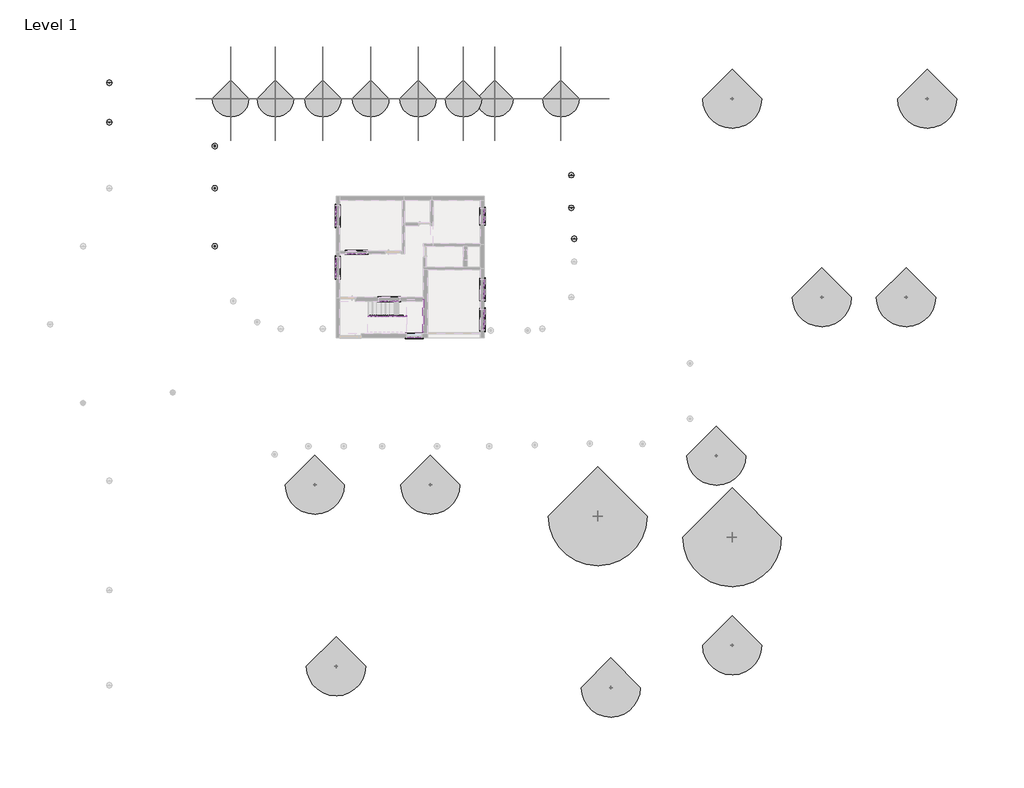
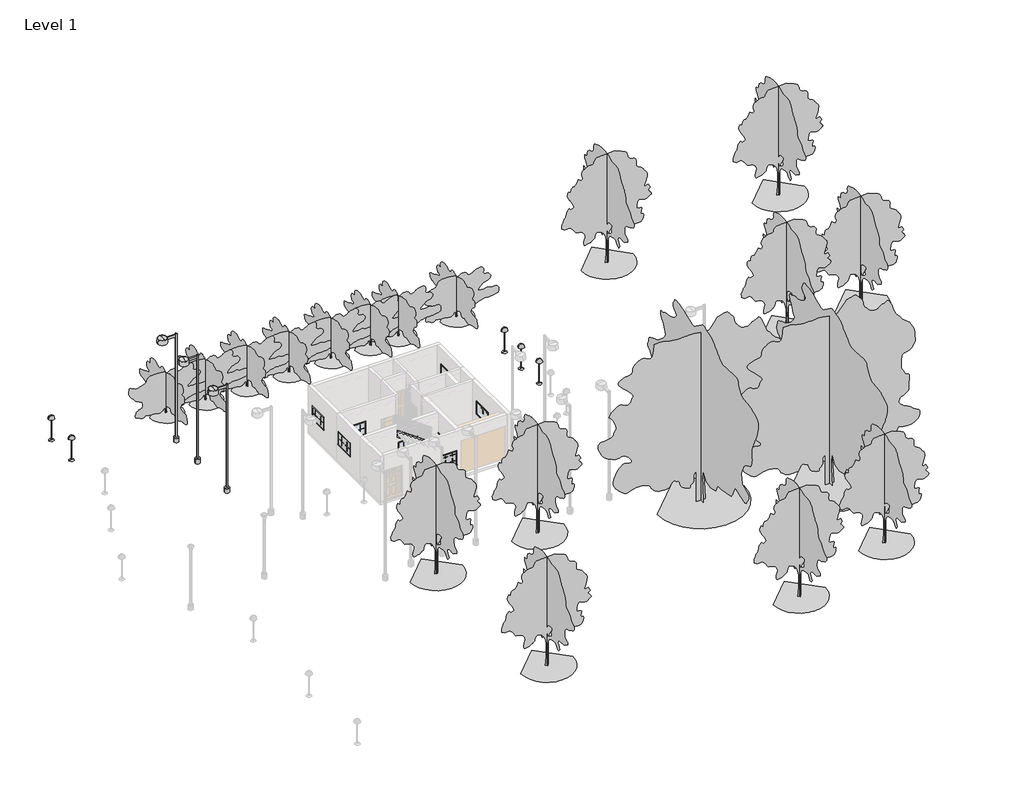
# One storey, part 3 of 3: 36 proxies, 20 geographic elements, 8 light fixtures, 4 members.
"""IFC4 building model written with IfcOpenShell, lengths in millimetres."""

from ifc_helpers import new_model, si_unit, frame, origin, place, context, project, spatial, polyline, outline, extrude, transform, mapped, element, save
from components import m_muntin_pattern_2x2_m_muntin_pattern_2x2_8d9e5da3, m_muntin_pattern_2x2_m_muntin_pattern_2x2_32a0f80e, m_muntin_pattern_2x2_m_muntin_pattern_2x2_5c9fa27a, m_muntin_pattern_2x2_m_muntin_pattern_2x2_8c7fd3cb, m_muntin_pattern_2x2_m_muntin_pattern_2x2_332c70e0, m_trim_window_exterior_flat_with_sill_3a557199, m_trim_window_exterior_flat_with_sill_8fa486dc, m_trim_window_interior_flat_picture_frame_580345df, m_trim_window_interior_flat_picture_frame_b6dd03a6, m_rpc_tree_deciduous_kousa_dogwood_3_0_meters_e0625334, m_rpc_tree_deciduous_largetooth_aspen_7_6_meters_a2efc43f, m_rpc_tree_deciduous_scarlet_oak_12_5_meters_78a4568a, m_floor_lamp_hemispheric_60w_120v_4a08ccbb, m_street_light_standard_250w_halogen_480v_204dbcbb

model = new_model("IFC4")

# Units and contexts
model_context = context("Model", 3, world=origin())
ifc_project = project(units=[si_unit("LENGTHUNIT", "METRE", prefix="MILLI")], contexts=[model_context])

# Site, building, storey
site = spatial("IfcSite", under=ifc_project)
building = spatial("IfcBuilding", under=site)
storey = spatial("IfcBuildingStorey", under=building, Name="Level 1", Elevation=0.0)

# Proxies
placement = place(None, origin())
m_muntin_pattern_2x2_m_muntin_pattern_2x2_shape = m_muntin_pattern_2x2_m_muntin_pattern_2x2_8d9e5da3(model_context)
element("IfcBuildingElementProxy", 1, Name="M_Muntin Pattern_2x2 : M_Muntin Pattern_2x2", ObjectType="M_Muntin Pattern_2x2 : M_Muntin Pattern_2x2", at=placement, inside=storey, context=model_context, shape_type="MappedRepresentation", body=[
    mapped(m_muntin_pattern_2x2_m_muntin_pattern_2x2_shape, transform((-8281.8157945, -2418.5171603, 1289.05), x_axis=(-1.0, 0.0, 0.0), y_axis=(0.0, -1.0, 0.0), z_axis=(0.0, 0.0, 1.0))),
])
element("IfcBuildingElementProxy", 2, Name="M_Muntin Pattern_2x2 : M_Muntin Pattern_2x2", ObjectType="M_Muntin Pattern_2x2 : M_Muntin Pattern_2x2", at=placement, inside=storey, context=model_context, shape_type="MappedRepresentation", body=[
    mapped(m_muntin_pattern_2x2_m_muntin_pattern_2x2_shape, transform((-3082.7532945, -3204.3296603, 1289.05), x_axis=(0.0, -1.0, 0.0), y_axis=(1.0, 0.0, 0.0), z_axis=(0.0, 0.0, 1.0))),
])
element("IfcBuildingElementProxy", 3, Name="M_Muntin Pattern_2x2 : M_Muntin Pattern_2x2", ObjectType="M_Muntin Pattern_2x2 : M_Muntin Pattern_2x2", at=placement, inside=storey, context=model_context, shape_type="MappedRepresentation", body=[
    mapped(m_muntin_pattern_2x2_m_muntin_pattern_2x2_shape, transform((-3082.7532945, -1461.6515353, 1289.05), x_axis=(0.0, -1.0, 0.0), y_axis=(1.0, 0.0, 0.0), z_axis=(0.0, 0.0, 1.0))),
])
element("IfcBuildingElementProxy", 4, Name="M_Muntin Pattern_2x2 : M_Muntin Pattern_2x2", ObjectType="M_Muntin Pattern_2x2 : M_Muntin Pattern_2x2", at=placement, inside=storey, context=model_context, shape_type="MappedRepresentation", body=[
    mapped(m_muntin_pattern_2x2_m_muntin_pattern_2x2_shape, transform((-11648.9032945, 2196.3453397, 1289.05), x_axis=(0.0, 1.0, 0.0), y_axis=(-1.0, 0.0, 0.0), z_axis=(0.0, 0.0, 1.0))),
])
element("IfcBuildingElementProxy", 5, Name="M_Muntin Pattern_2x2 : M_Muntin Pattern_2x2", ObjectType="M_Muntin Pattern_2x2 : M_Muntin Pattern_2x2", at=placement, inside=storey, context=model_context, shape_type="MappedRepresentation", body=[
    mapped(m_muntin_pattern_2x2_m_muntin_pattern_2x2_shape, transform((-11648.9032945, -800.8546603, 1289.05), x_axis=(0.0, 1.0, 0.0), y_axis=(-1.0, 0.0, 0.0), z_axis=(0.0, 0.0, 1.0))),
])
element("IfcBuildingElementProxy", 6, Name="M_Muntin Pattern_2x2 : M_Muntin Pattern_2x2", ObjectType="M_Muntin Pattern_2x2 : M_Muntin Pattern_2x2", at=placement, inside=storey, context=model_context, shape_type="MappedRepresentation", body=[
    mapped(m_muntin_pattern_2x2_m_muntin_pattern_2x2_shape, transform((-10165.3845445, 324.6828397, 1289.05), x_axis=(-1.0, 0.0, 0.0), y_axis=(0.0, -1.0, 0.0), z_axis=(0.0, 0.0, 1.0))),
])
m_muntin_pattern_2x2_m_muntin_pattern_2x2_2_shape = m_muntin_pattern_2x2_m_muntin_pattern_2x2_32a0f80e(model_context)
element("IfcBuildingElementProxy", 7, Name="M_Muntin Pattern_2x2 : M_Muntin Pattern_2x2", ObjectType="M_Muntin Pattern_2x2 : M_Muntin Pattern_2x2", at=placement, inside=storey, context=model_context, shape_type="MappedRepresentation", body=[
    mapped(m_muntin_pattern_2x2_m_muntin_pattern_2x2_2_shape, transform((-8888.2407945, -2418.5171603, 1289.05), x_axis=(1.0, 0.0, 0.0), y_axis=(0.0, 1.0, 0.0), z_axis=(0.0, 0.0, 1.0))),
])
element("IfcBuildingElementProxy", 8, Name="M_Muntin Pattern_2x2 : M_Muntin Pattern_2x2", ObjectType="M_Muntin Pattern_2x2 : M_Muntin Pattern_2x2", at=placement, inside=storey, context=model_context, shape_type="MappedRepresentation", body=[
    mapped(m_muntin_pattern_2x2_m_muntin_pattern_2x2_2_shape, transform((-3082.7532945, -3810.7546603, 1289.05), x_axis=(0.0, 1.0, 0.0), y_axis=(-1.0, 0.0, 0.0), z_axis=(0.0, 0.0, 1.0))),
])
element("IfcBuildingElementProxy", 9, Name="M_Muntin Pattern_2x2 : M_Muntin Pattern_2x2", ObjectType="M_Muntin Pattern_2x2 : M_Muntin Pattern_2x2", at=placement, inside=storey, context=model_context, shape_type="MappedRepresentation", body=[
    mapped(m_muntin_pattern_2x2_m_muntin_pattern_2x2_2_shape, transform((-3082.7532945, -2068.0765353, 1289.05), x_axis=(0.0, 1.0, 0.0), y_axis=(-1.0, 0.0, 0.0), z_axis=(0.0, 0.0, 1.0))),
])
element("IfcBuildingElementProxy", 10, Name="M_Muntin Pattern_2x2 : M_Muntin Pattern_2x2", ObjectType="M_Muntin Pattern_2x2 : M_Muntin Pattern_2x2", at=placement, inside=storey, context=model_context, shape_type="MappedRepresentation", body=[
    mapped(m_muntin_pattern_2x2_m_muntin_pattern_2x2_2_shape, transform((-11648.9032945, 2802.7703397, 1289.05), x_axis=(0.0, -1.0, 0.0), y_axis=(1.0, 0.0, 0.0), z_axis=(0.0, 0.0, 1.0))),
])
element("IfcBuildingElementProxy", 11, Name="M_Muntin Pattern_2x2 : M_Muntin Pattern_2x2", ObjectType="M_Muntin Pattern_2x2 : M_Muntin Pattern_2x2", at=placement, inside=storey, context=model_context, shape_type="MappedRepresentation", body=[
    mapped(m_muntin_pattern_2x2_m_muntin_pattern_2x2_2_shape, transform((-11648.9032945, -194.4296603, 1289.05), x_axis=(0.0, -1.0, 0.0), y_axis=(1.0, 0.0, 0.0), z_axis=(0.0, 0.0, 1.0))),
])
element("IfcBuildingElementProxy", 12, Name="M_Muntin Pattern_2x2 : M_Muntin Pattern_2x2", ObjectType="M_Muntin Pattern_2x2 : M_Muntin Pattern_2x2", at=placement, inside=storey, context=model_context, shape_type="MappedRepresentation", body=[
    mapped(m_muntin_pattern_2x2_m_muntin_pattern_2x2_2_shape, transform((-10771.8095445, 324.6828397, 1289.05), x_axis=(1.0, 0.0, 0.0), y_axis=(0.0, 1.0, 0.0), z_axis=(0.0, 0.0, 1.0))),
])
m_muntin_pattern_2x2_m_muntin_pattern_2x2_3_shape = m_muntin_pattern_2x2_m_muntin_pattern_2x2_5c9fa27a(model_context)
element("IfcBuildingElementProxy", 13, Name="M_Muntin Pattern_2x2 : M_Muntin Pattern_2x2", ObjectType="M_Muntin Pattern_2x2 : M_Muntin Pattern_2x2", at=placement, inside=storey, context=model_context, shape_type="MappedRepresentation", body=[
    mapped(m_muntin_pattern_2x2_m_muntin_pattern_2x2_3_shape, transform((-6910.2157945, -4552.1171603, 984.25), x_axis=(-1.0, 0.0, 0.0), y_axis=(0.0, -1.0, 0.0), z_axis=(0.0, 0.0, 1.0))),
])
element("IfcBuildingElementProxy", 14, Name="M_Muntin Pattern_2x2 : M_Muntin Pattern_2x2", ObjectType="M_Muntin Pattern_2x2 : M_Muntin Pattern_2x2", at=placement, inside=storey, context=model_context, shape_type="MappedRepresentation", body=[
    mapped(m_muntin_pattern_2x2_m_muntin_pattern_2x2_3_shape, transform((-3082.7532945, 2701.1703397, 1289.05), x_axis=(0.0, -1.0, 0.0), y_axis=(1.0, 0.0, 0.0), z_axis=(0.0, 0.0, 1.0))),
])
m_muntin_pattern_2x2_m_muntin_pattern_2x2_4_shape = m_muntin_pattern_2x2_m_muntin_pattern_2x2_8c7fd3cb(model_context)
element("IfcBuildingElementProxy", 15, Name="M_Muntin Pattern_2x2 : M_Muntin Pattern_2x2", ObjectType="M_Muntin Pattern_2x2 : M_Muntin Pattern_2x2", at=placement, inside=storey, context=model_context, shape_type="MappedRepresentation", body=[
    mapped(m_muntin_pattern_2x2_m_muntin_pattern_2x2_4_shape, transform((-7364.2407945, -4552.1171603, 984.25), x_axis=(1.0, 0.0, 0.0), y_axis=(0.0, 1.0, 0.0), z_axis=(0.0, 0.0, 1.0))),
])
element("IfcBuildingElementProxy", 16, Name="M_Muntin Pattern_2x2 : M_Muntin Pattern_2x2", ObjectType="M_Muntin Pattern_2x2 : M_Muntin Pattern_2x2", at=placement, inside=storey, context=model_context, shape_type="MappedRepresentation", body=[
    mapped(m_muntin_pattern_2x2_m_muntin_pattern_2x2_4_shape, transform((-3082.7532945, 2247.1453397, 1289.05), x_axis=(0.0, 1.0, 0.0), y_axis=(-1.0, 0.0, 0.0), z_axis=(0.0, 0.0, 1.0))),
])
m_muntin_pattern_2x2_m_muntin_pattern_2x2_5_shape = m_muntin_pattern_2x2_m_muntin_pattern_2x2_332c70e0(model_context)
element("IfcBuildingElementProxy", 17, Name="M_Muntin Pattern_2x2 : M_Muntin Pattern_2x2", ObjectType="M_Muntin Pattern_2x2 : M_Muntin Pattern_2x2", at=placement, inside=storey, context=model_context, shape_type="MappedRepresentation", body=[
    mapped(m_muntin_pattern_2x2_m_muntin_pattern_2x2_5_shape, transform((-7364.2407945, -4552.1171603, 1584.25), x_axis=(1.0, 0.0, 0.0), y_axis=(0.0, 1.0, 0.0), z_axis=(0.0, 0.0, 1.0))),
])
element("IfcBuildingElementProxy", 18, Name="M_Muntin Pattern_2x2 : M_Muntin Pattern_2x2", ObjectType="M_Muntin Pattern_2x2 : M_Muntin Pattern_2x2", at=placement, inside=storey, context=model_context, shape_type="MappedRepresentation", body=[
    mapped(m_muntin_pattern_2x2_m_muntin_pattern_2x2_5_shape, transform((-6910.2157945, -4552.1171603, 1584.25), x_axis=(1.0, 0.0, 0.0), y_axis=(0.0, 1.0, 0.0), z_axis=(0.0, 0.0, 1.0))),
])
element("IfcBuildingElementProxy", 19, Name="M_Muntin Pattern_2x2 : M_Muntin Pattern_2x2", ObjectType="M_Muntin Pattern_2x2 : M_Muntin Pattern_2x2", at=placement, inside=storey, context=model_context, shape_type="MappedRepresentation", body=[
    mapped(m_muntin_pattern_2x2_m_muntin_pattern_2x2_5_shape, transform((-3082.7532945, 2247.1453397, 1889.05), x_axis=(0.0, 1.0, 0.0), y_axis=(-1.0, 0.0, 0.0), z_axis=(0.0, 0.0, 1.0))),
])
element("IfcBuildingElementProxy", 20, Name="M_Muntin Pattern_2x2 : M_Muntin Pattern_2x2", ObjectType="M_Muntin Pattern_2x2 : M_Muntin Pattern_2x2", at=placement, inside=storey, context=model_context, shape_type="MappedRepresentation", body=[
    mapped(m_muntin_pattern_2x2_m_muntin_pattern_2x2_5_shape, transform((-3082.7532945, 2701.1703397, 1889.05), x_axis=(0.0, 1.0, 0.0), y_axis=(-1.0, 0.0, 0.0), z_axis=(0.0, 0.0, 1.0))),
])
m_trim_window_exterior_flat_with_sill_shape = m_trim_window_exterior_flat_with_sill_3a557199(model_context)
element("IfcBuildingElementProxy", 21, Name="M_Trim-Window-Exterior-Flat : with Sill", ObjectType="M_Trim-Window-Exterior-Flat : with Sill", at=placement, inside=storey, context=model_context, shape_type="MappedRepresentation", body=[
    mapped(m_trim_window_exterior_flat_with_sill_shape, transform((-8585.0282945, -2428.0421603, 2019.2), x_axis=(1.0, 0.0, 0.0), y_axis=(0.0, 0.0, 1.0), z_axis=(0.0, -1.0, 0.0))),
])
element("IfcBuildingElementProxy", 22, Name="M_Trim-Window-Exterior-Flat : with Sill", ObjectType="M_Trim-Window-Exterior-Flat : with Sill", at=placement, inside=storey, context=model_context, shape_type="MappedRepresentation", body=[
    mapped(m_trim_window_exterior_flat_with_sill_shape, transform((-3073.2282945, -3507.5421603, 2019.2), x_axis=(0.0, 1.0, 0.0), y_axis=(0.0, 0.0, 1.0), z_axis=(1.0, 0.0, 0.0))),
])
element("IfcBuildingElementProxy", 23, Name="M_Trim-Window-Exterior-Flat : with Sill", ObjectType="M_Trim-Window-Exterior-Flat : with Sill", at=placement, inside=storey, context=model_context, shape_type="MappedRepresentation", body=[
    mapped(m_trim_window_exterior_flat_with_sill_shape, transform((-3073.2282945, -1764.8640353, 2019.2), x_axis=(0.0, 1.0, 0.0), y_axis=(0.0, 0.0, 1.0), z_axis=(1.0, 0.0, 0.0))),
])
element("IfcBuildingElementProxy", 24, Name="M_Trim-Window-Exterior-Flat : with Sill", ObjectType="M_Trim-Window-Exterior-Flat : with Sill", at=placement, inside=storey, context=model_context, shape_type="MappedRepresentation", body=[
    mapped(m_trim_window_exterior_flat_with_sill_shape, transform((-11658.4282945, 2499.5578397, 2019.2), x_axis=(0.0, -1.0, 0.0), y_axis=(0.0, 0.0, 1.0), z_axis=(-1.0, 0.0, 0.0))),
])
element("IfcBuildingElementProxy", 25, Name="M_Trim-Window-Exterior-Flat : with Sill", ObjectType="M_Trim-Window-Exterior-Flat : with Sill", at=placement, inside=storey, context=model_context, shape_type="MappedRepresentation", body=[
    mapped(m_trim_window_exterior_flat_with_sill_shape, transform((-11658.4282945, -497.6421603, 2019.2), x_axis=(0.0, -1.0, 0.0), y_axis=(0.0, 0.0, 1.0), z_axis=(-1.0, 0.0, 0.0))),
])
element("IfcBuildingElementProxy", 26, Name="M_Trim-Window-Exterior-Flat : with Sill", ObjectType="M_Trim-Window-Exterior-Flat : with Sill", at=placement, inside=storey, context=model_context, shape_type="MappedRepresentation", body=[
    mapped(m_trim_window_exterior_flat_with_sill_shape, transform((-10468.5970445, 315.1578397, 2019.2), x_axis=(1.0, 0.0, 0.0), y_axis=(0.0, 0.0, 1.0), z_axis=(0.0, -1.0, 0.0))),
])
m_trim_window_exterior_flat_with_sill_2_shape = m_trim_window_exterior_flat_with_sill_8fa486dc(model_context)
element("IfcBuildingElementProxy", 27, Name="M_Trim-Window-Exterior-Flat : with Sill", ObjectType="M_Trim-Window-Exterior-Flat : with Sill", at=placement, inside=storey, context=model_context, shape_type="MappedRepresentation", body=[
    mapped(m_trim_window_exterior_flat_with_sill_2_shape, transform((-7137.2282945, -4561.6421603, 1814.4), x_axis=(1.0, 0.0, 0.0), y_axis=(0.0, 0.0, 1.0), z_axis=(0.0, -1.0, 0.0))),
])
element("IfcBuildingElementProxy", 28, Name="M_Trim-Window-Exterior-Flat : with Sill", ObjectType="M_Trim-Window-Exterior-Flat : with Sill", at=placement, inside=storey, context=model_context, shape_type="MappedRepresentation", body=[
    mapped(m_trim_window_exterior_flat_with_sill_2_shape, transform((-3073.2282945, 2474.1578397, 2119.2), x_axis=(0.0, 1.0, 0.0), y_axis=(0.0, 0.0, 1.0), z_axis=(1.0, 0.0, 0.0))),
])
m_trim_window_interior_flat_picture_frame_shape = m_trim_window_interior_flat_picture_frame_580345df(model_context)
element("IfcBuildingElementProxy", 29, Name="M_Trim-Window-Interior-Flat : Picture Frame", ObjectType="M_Trim-Window-Interior-Flat : Picture Frame", at=placement, inside=storey, context=model_context, shape_type="MappedRepresentation", body=[
    mapped(m_trim_window_interior_flat_picture_frame_shape, transform((-8585.0282945, -2199.4421603, 2019.2), x_axis=(-1.0, 0.0, 0.0), y_axis=(0.0, 0.0, 1.0), z_axis=(0.0, 1.0, 0.0))),
])
element("IfcBuildingElementProxy", 30, Name="M_Trim-Window-Interior-Flat : Picture Frame", ObjectType="M_Trim-Window-Interior-Flat : Picture Frame", at=placement, inside=storey, context=model_context, shape_type="MappedRepresentation", body=[
    mapped(m_trim_window_interior_flat_picture_frame_shape, transform((-3301.8282945, -3507.5421603, 2019.2), x_axis=(0.0, -1.0, 0.0), y_axis=(0.0, 0.0, 1.0), z_axis=(-1.0, 0.0, 0.0))),
])
element("IfcBuildingElementProxy", 31, Name="M_Trim-Window-Interior-Flat : Picture Frame", ObjectType="M_Trim-Window-Interior-Flat : Picture Frame", at=placement, inside=storey, context=model_context, shape_type="MappedRepresentation", body=[
    mapped(m_trim_window_interior_flat_picture_frame_shape, transform((-3301.8282945, -1764.8640353, 2019.2), x_axis=(0.0, -1.0, 0.0), y_axis=(0.0, 0.0, 1.0), z_axis=(-1.0, 0.0, 0.0))),
])
element("IfcBuildingElementProxy", 32, Name="M_Trim-Window-Interior-Flat : Picture Frame", ObjectType="M_Trim-Window-Interior-Flat : Picture Frame", at=placement, inside=storey, context=model_context, shape_type="MappedRepresentation", body=[
    mapped(m_trim_window_interior_flat_picture_frame_shape, transform((-11429.8282945, 2499.5578397, 2019.2), x_axis=(0.0, 1.0, 0.0), y_axis=(0.0, 0.0, 1.0), z_axis=(1.0, 0.0, 0.0))),
])
element("IfcBuildingElementProxy", 33, Name="M_Trim-Window-Interior-Flat : Picture Frame", ObjectType="M_Trim-Window-Interior-Flat : Picture Frame", at=placement, inside=storey, context=model_context, shape_type="MappedRepresentation", body=[
    mapped(m_trim_window_interior_flat_picture_frame_shape, transform((-11429.8282945, -497.6421603, 2019.2), x_axis=(0.0, 1.0, 0.0), y_axis=(0.0, 0.0, 1.0), z_axis=(1.0, 0.0, 0.0))),
])
element("IfcBuildingElementProxy", 34, Name="M_Trim-Window-Interior-Flat : Picture Frame", ObjectType="M_Trim-Window-Interior-Flat : Picture Frame", at=placement, inside=storey, context=model_context, shape_type="MappedRepresentation", body=[
    mapped(m_trim_window_interior_flat_picture_frame_shape, transform((-10468.5970445, 467.5578397, 2019.2), x_axis=(-1.0, 0.0, 0.0), y_axis=(0.0, 0.0, 1.0), z_axis=(0.0, 1.0, 0.0))),
])
m_trim_window_interior_flat_picture_frame_2_shape = m_trim_window_interior_flat_picture_frame_b6dd03a6(model_context)
element("IfcBuildingElementProxy", 35, Name="M_Trim-Window-Interior-Flat : Picture Frame", ObjectType="M_Trim-Window-Interior-Flat : Picture Frame", at=placement, inside=storey, context=model_context, shape_type="MappedRepresentation", body=[
    mapped(m_trim_window_interior_flat_picture_frame_2_shape, transform((-7137.2282945, -4333.0421603, 1814.4), x_axis=(-1.0, 0.0, 0.0), y_axis=(0.0, 0.0, 1.0), z_axis=(0.0, 1.0, 0.0))),
])
element("IfcBuildingElementProxy", 36, Name="M_Trim-Window-Interior-Flat : Picture Frame", ObjectType="M_Trim-Window-Interior-Flat : Picture Frame", at=placement, inside=storey, context=model_context, shape_type="MappedRepresentation", body=[
    mapped(m_trim_window_interior_flat_picture_frame_2_shape, transform((-3301.8282945, 2474.1578397, 2119.2), x_axis=(0.0, -1.0, 0.0), y_axis=(0.0, 0.0, 1.0), z_axis=(-1.0, 0.0, 0.0))),
])

# Geographic elements
m_rpc_tree_deciduous_kousa_dogwood_3_0_meters_shape = m_rpc_tree_deciduous_kousa_dogwood_3_0_meters_e0625334(model_context)
element("IfcGeographicElement", 37, ObjectType="M_RPC Tree - Deciduous : Kousa Dogwood - 3.0 Meters", at=placement, inside=storey, context=model_context, shape_type="MappedRepresentation", body=[
    mapped(m_rpc_tree_deciduous_kousa_dogwood_3_0_meters_shape, transform((-17754.4282945, 9281.3578397, 0.0), x_axis=(1.0, 0.0, 0.0), y_axis=(0.0, 1.0, 0.0), z_axis=(0.0, 0.0, 1.0))),
])
element("IfcGeographicElement", 38, ObjectType="M_RPC Tree - Deciduous : Kousa Dogwood - 3.0 Meters", at=placement, inside=storey, context=model_context, shape_type="MappedRepresentation", body=[
    mapped(m_rpc_tree_deciduous_kousa_dogwood_3_0_meters_shape, transform((-15163.6282945, 9281.3578397, 0.0), x_axis=(1.0, 0.0, 0.0), y_axis=(0.0, 1.0, 0.0), z_axis=(0.0, 0.0, 1.0))),
])
element("IfcGeographicElement", 39, ObjectType="M_RPC Tree - Deciduous : Kousa Dogwood - 3.0 Meters", at=placement, inside=storey, context=model_context, shape_type="MappedRepresentation", body=[
    mapped(m_rpc_tree_deciduous_kousa_dogwood_3_0_meters_shape, transform((-12420.4282945, 9281.3578397, 0.0), x_axis=(1.0, 0.0, 0.0), y_axis=(0.0, 1.0, 0.0), z_axis=(0.0, 0.0, 1.0))),
])
element("IfcGeographicElement", 40, ObjectType="M_RPC Tree - Deciduous : Kousa Dogwood - 3.0 Meters", at=placement, inside=storey, context=model_context, shape_type="MappedRepresentation", body=[
    mapped(m_rpc_tree_deciduous_kousa_dogwood_3_0_meters_shape, transform((-9651.8282945, 9281.3578397, 0.0), x_axis=(1.0, 0.0, 0.0), y_axis=(0.0, 1.0, 0.0), z_axis=(0.0, 0.0, 1.0))),
])
element("IfcGeographicElement", 41, ObjectType="M_RPC Tree - Deciduous : Kousa Dogwood - 3.0 Meters", at=placement, inside=storey, context=model_context, shape_type="MappedRepresentation", body=[
    mapped(m_rpc_tree_deciduous_kousa_dogwood_3_0_meters_shape, transform((-6908.6282945, 9281.3578397, 0.0), x_axis=(1.0, 0.0, 0.0), y_axis=(0.0, 1.0, 0.0), z_axis=(0.0, 0.0, 1.0))),
])
element("IfcGeographicElement", 42, ObjectType="M_RPC Tree - Deciduous : Kousa Dogwood - 3.0 Meters", at=placement, inside=storey, context=model_context, shape_type="MappedRepresentation", body=[
    mapped(m_rpc_tree_deciduous_kousa_dogwood_3_0_meters_shape, transform((-2463.6282945, 9281.3578397, 0.0), x_axis=(1.0, 0.0, 0.0), y_axis=(0.0, 1.0, 0.0), z_axis=(0.0, 0.0, 1.0))),
])
element("IfcGeographicElement", 43, ObjectType="M_RPC Tree - Deciduous : Kousa Dogwood - 3.0 Meters", at=placement, inside=storey, context=model_context, shape_type="MappedRepresentation", body=[
    mapped(m_rpc_tree_deciduous_kousa_dogwood_3_0_meters_shape, transform((1346.3717055, 9281.3578397, 0.0), x_axis=(1.0, 0.0, 0.0), y_axis=(0.0, 1.0, 0.0), z_axis=(0.0, 0.0, 1.0))),
])
element("IfcGeographicElement", 44, ObjectType="M_RPC Tree - Deciduous : Kousa Dogwood - 3.0 Meters", at=placement, inside=storey, context=model_context, shape_type="MappedRepresentation", body=[
    mapped(m_rpc_tree_deciduous_kousa_dogwood_3_0_meters_shape, transform((-4292.4282945, 9281.3578397, 0.0), x_axis=(1.0, 0.0, 0.0), y_axis=(0.0, 1.0, 0.0), z_axis=(0.0, 0.0, 1.0))),
])
m_rpc_tree_deciduous_largetooth_aspen_7_6_meters_shape = m_rpc_tree_deciduous_largetooth_aspen_7_6_meters_a2efc43f(model_context)
element("IfcGeographicElement", 45, ObjectType="M_RPC Tree - Deciduous : Largetooth Aspen - 7.6 Meters", at=placement, inside=storey, context=model_context, shape_type="MappedRepresentation", body=[
    mapped(m_rpc_tree_deciduous_largetooth_aspen_7_6_meters_shape, transform((-12877.6282945, -13045.2421603, 637.7976981), x_axis=(1.0, 0.0, 0.0), y_axis=(0.0, 1.0, 0.0), z_axis=(0.0, 0.0, 1.0))),
])
element("IfcGeographicElement", 46, ObjectType="M_RPC Tree - Deciduous : Largetooth Aspen - 7.6 Meters", at=placement, inside=storey, context=model_context, shape_type="MappedRepresentation", body=[
    mapped(m_rpc_tree_deciduous_largetooth_aspen_7_6_meters_shape, transform((-6197.4282945, -13045.2421603, 1145.9723708), x_axis=(1.0, 0.0, 0.0), y_axis=(0.0, 1.0, 0.0), z_axis=(0.0, 0.0, 1.0))),
])
element("IfcGeographicElement", 47, ObjectType="M_RPC Tree - Deciduous : Largetooth Aspen - 7.6 Meters", at=placement, inside=storey, context=model_context, shape_type="MappedRepresentation", body=[
    mapped(m_rpc_tree_deciduous_largetooth_aspen_7_6_meters_shape, transform((10337.9717055, -11368.7940322, 23.6768758), x_axis=(1.0, 0.0, 0.0), y_axis=(0.0, 1.0, 0.0), z_axis=(0.0, 0.0, 1.0))),
])
element("IfcGeographicElement", 48, ObjectType="M_RPC Tree - Deciduous : Largetooth Aspen - 7.6 Meters", at=placement, inside=storey, context=model_context, shape_type="MappedRepresentation", body=[
    mapped(m_rpc_tree_deciduous_largetooth_aspen_7_6_meters_shape, transform((-11658.4282945, -23560.8421603, 216.6633849), x_axis=(1.0, 0.0, 0.0), y_axis=(0.0, 1.0, 0.0), z_axis=(0.0, 0.0, 1.0))),
])
element("IfcGeographicElement", 49, ObjectType="M_RPC Tree - Deciduous : Largetooth Aspen - 7.6 Meters", at=placement, inside=storey, context=model_context, shape_type="MappedRepresentation", body=[
    mapped(m_rpc_tree_deciduous_largetooth_aspen_7_6_meters_shape, transform((4241.9717055, -24780.0421603, 189.5016682), x_axis=(1.0, 0.0, 0.0), y_axis=(0.0, 1.0, 0.0), z_axis=(0.0, 0.0, 1.0))),
])
element("IfcGeographicElement", 50, ObjectType="M_RPC Tree - Deciduous : Largetooth Aspen - 7.6 Meters", at=placement, inside=storey, context=model_context, shape_type="MappedRepresentation", body=[
    mapped(m_rpc_tree_deciduous_largetooth_aspen_7_6_meters_shape, transform((11252.3717055, -22341.6421603, 0.0), x_axis=(1.0, 0.0, 0.0), y_axis=(0.0, 1.0, 0.0), z_axis=(0.0, 0.0, 1.0))),
])
element("IfcGeographicElement", 51, ObjectType="M_RPC Tree - Deciduous : Largetooth Aspen - 7.6 Meters", at=placement, inside=storey, context=model_context, shape_type="MappedRepresentation", body=[
    mapped(m_rpc_tree_deciduous_largetooth_aspen_7_6_meters_shape, transform((21310.7717055, -2199.4421603, 830.3815922), x_axis=(1.0, 0.0, 0.0), y_axis=(0.0, 1.0, 0.0), z_axis=(0.0, 0.0, 1.0))),
])
element("IfcGeographicElement", 52, ObjectType="M_RPC Tree - Deciduous : Largetooth Aspen - 7.6 Meters", at=placement, inside=storey, context=model_context, shape_type="MappedRepresentation", body=[
    mapped(m_rpc_tree_deciduous_largetooth_aspen_7_6_meters_shape, transform((16445.6374905, -2199.4421603, 708.9278868), x_axis=(1.0, 0.0, 0.0), y_axis=(0.0, 1.0, 0.0), z_axis=(0.0, 0.0, 1.0))),
])
element("IfcGeographicElement", 53, ObjectType="M_RPC Tree - Deciduous : Largetooth Aspen - 7.6 Meters", at=placement, inside=storey, context=model_context, shape_type="MappedRepresentation", body=[
    mapped(m_rpc_tree_deciduous_largetooth_aspen_7_6_meters_shape, transform((11252.3717055, 9281.3578397, 321.1951869), x_axis=(1.0, 0.0, 0.0), y_axis=(0.0, 1.0, 0.0), z_axis=(0.0, 0.0, 1.0))),
])
element("IfcGeographicElement", 54, ObjectType="M_RPC Tree - Deciduous : Largetooth Aspen - 7.6 Meters", at=placement, inside=storey, context=model_context, shape_type="MappedRepresentation", body=[
    mapped(m_rpc_tree_deciduous_largetooth_aspen_7_6_meters_shape, transform((22529.9717055, 9281.3578397, 1067.3341196), x_axis=(1.0, 0.0, 0.0), y_axis=(0.0, 1.0, 0.0), z_axis=(0.0, 0.0, 1.0))),
])
m_rpc_tree_deciduous_scarlet_oak_12_5_meters_shape = m_rpc_tree_deciduous_scarlet_oak_12_5_meters_78a4568a(model_context)
element("IfcGeographicElement", 55, ObjectType="M_RPC Tree - Deciduous : Scarlet Oak - 12.5 Meters", at=placement, inside=storey, context=model_context, shape_type="MappedRepresentation", body=[
    mapped(m_rpc_tree_deciduous_scarlet_oak_12_5_meters_shape, transform((3479.9717055, -14874.0421603, 1128.9992751), x_axis=(1.0, 0.0, 0.0), y_axis=(0.0, 1.0, 0.0), z_axis=(0.0, 0.0, 1.0))),
])
element("IfcGeographicElement", 56, ObjectType="M_RPC Tree - Deciduous : Scarlet Oak - 12.5 Meters", at=placement, inside=storey, context=model_context, shape_type="MappedRepresentation", body=[
    mapped(m_rpc_tree_deciduous_scarlet_oak_12_5_meters_shape, transform((11252.3717055, -16093.2421603, 316.4414862), x_axis=(1.0, 0.0, 0.0), y_axis=(0.0, 1.0, 0.0), z_axis=(0.0, 0.0, 1.0))),
])

# Light fixtures
m_floor_lamp_hemispheric_60w_120v_shape = m_floor_lamp_hemispheric_60w_120v_4a08ccbb(model_context)
element("IfcLightFixture", 57, ObjectType="M_Floor Lamp - Hemispheric : 60W - 120V", at=placement, inside=storey, context=model_context, shape_type="MappedRepresentation", body=[
    mapped(m_floor_lamp_hemispheric_60w_120v_shape, transform((-24764.8282945, 10195.7578397, 0.0), x_axis=(1.0, 0.0, 0.0), y_axis=(0.0, 1.0, 0.0), z_axis=(0.0, 0.0, 1.0))),
])
element("IfcLightFixture", 58, ObjectType="M_Floor Lamp - Hemispheric : 60W - 120V", at=placement, inside=storey, context=model_context, shape_type="MappedRepresentation", body=[
    mapped(m_floor_lamp_hemispheric_60w_120v_shape, transform((-24764.8282945, 7909.7578397, 0.0), x_axis=(1.0, 0.0, 0.0), y_axis=(0.0, 1.0, 0.0), z_axis=(0.0, 0.0, 1.0))),
])
element("IfcLightFixture", 59, ObjectType="M_Floor Lamp - Hemispheric : 60W - 120V", at=placement, inside=storey, context=model_context, shape_type="MappedRepresentation", body=[
    mapped(m_floor_lamp_hemispheric_60w_120v_shape, transform((1955.9717055, 4861.7578397, 0.0), x_axis=(1.0, 0.0, 0.0), y_axis=(0.0, 1.0, 0.0), z_axis=(0.0, 0.0, 1.0))),
])
element("IfcLightFixture", 60, ObjectType="M_Floor Lamp - Hemispheric : 60W - 120V", at=placement, inside=storey, context=model_context, shape_type="MappedRepresentation", body=[
    mapped(m_floor_lamp_hemispheric_60w_120v_shape, transform((1955.9717055, 2956.7578397, 0.0), x_axis=(1.0, 0.0, 0.0), y_axis=(0.0, 1.0, 0.0), z_axis=(0.0, 0.0, 1.0))),
])
element("IfcLightFixture", 61, ObjectType="M_Floor Lamp - Hemispheric : 60W - 120V", at=placement, inside=storey, context=model_context, shape_type="MappedRepresentation", body=[
    mapped(m_floor_lamp_hemispheric_60w_120v_shape, transform((2108.3717055, 1178.7578397, 0.0), x_axis=(1.0, 0.0, 0.0), y_axis=(0.0, 1.0, 0.0), z_axis=(0.0, 0.0, 1.0))),
])
m_street_light_standard_250w_halogen_480v_shape = m_street_light_standard_250w_halogen_480v_204dbcbb(model_context)
element("IfcLightFixture", 62, ObjectType="M_Street Light - Standard : 400W Halogen - 120V", at=placement, inside=storey, context=model_context, shape_type="MappedRepresentation", body=[
    mapped(m_street_light_standard_250w_halogen_480v_shape, transform((-18668.8282945, 6538.1578397, 0.0), x_axis=(1.0, 0.0, 0.0), y_axis=(0.0, 1.0, 0.0), z_axis=(0.0, 0.0, 1.0))),
])
element("IfcLightFixture", 63, ObjectType="M_Street Light - Standard : 400W Halogen - 120V", at=placement, inside=storey, context=model_context, shape_type="MappedRepresentation", body=[
    mapped(m_street_light_standard_250w_halogen_480v_shape, transform((-18668.8282945, 4099.7578397, 0.0), x_axis=(1.0, 0.0, 0.0), y_axis=(0.0, 1.0, 0.0), z_axis=(0.0, 0.0, 1.0))),
])
element("IfcLightFixture", 64, ObjectType="M_Street Light - Standard : 400W Halogen - 120V", at=placement, inside=storey, context=model_context, shape_type="MappedRepresentation", body=[
    mapped(m_street_light_standard_250w_halogen_480v_shape, transform((-18668.8282945, 746.9578397, 0.0), x_axis=(1.0, 0.0, 0.0), y_axis=(0.0, 1.0, 0.0), z_axis=(0.0, 0.0, 1.0))),
])

# Members
element("IfcMember", 65, ObjectType="Stringer - 50mm Width", at=placement, inside=storey, context=model_context, shape_type="SweptSolid", body=[
    extrude(outline(polyline([(247.8881609, -9804.2282945), (0.0, -9804.2282945), (0.0, -9462.6128607), (1321.6831035, -7604.2282945), (1812.5281609, -7604.2282945), (247.8881609, -9804.2282945)])), frame((0.0, -3297.1921603, 0.0), z_axis=(0.0, 1.0, 0.0), x_axis=(0.0, 0.0, 1.0)), (0.0, 0.0, 1.0), 50.0),
])
element("IfcMember", 66, ObjectType="Stringer - 50mm Width", at=placement, inside=storey, context=model_context, shape_type="SweptSolid", body=[
    extrude(outline(polyline([(1535.0431035, -7554.2282945), (2025.8881609, -7554.2282945), (3626.0881609, -9804.2282945), (3135.2431035, -9804.2282945), (1535.0431035, -7554.2282945)])), frame((0.0, -3323.3921603, 0.0), z_axis=(0.0, 1.0, 0.0), x_axis=(0.0, 0.0, 1.0)), (0.0, 0.0, 1.0), 50.0),
])
element("IfcMember", 67, ObjectType="Stringer - 50mm Width", at=placement, inside=storey, context=model_context, shape_type="SweptSolid", body=[
    extrude(outline(polyline([(-6589.8282945, -4237.7921603), (-6639.8282945, -4237.7921603), (-6639.8282945, -2332.7921603), (-6589.8282945, -2332.7921603), (-6589.8282945, -4237.7921603)])), frame((0.0, 0.0, 1428.0), z_axis=(0.0, 0.0, 1.0), x_axis=(1.0, 0.0, 0.0)), (0.0, 0.0, 1.0), 400.0),
])
element("IfcMember", 68, ObjectType="Stringer - 50mm Width", at=placement, inside=storey, context=model_context, shape_type="SweptSolid", body=[
    extrude(outline(polyline([(-7604.2282945, -3247.1921603), (-7554.2282945, -3247.1921603), (-7554.2282945, -3273.3921603), (-7604.2282945, -3273.3921603), (-7604.2282945, -3247.1921603)])), frame((0.0, 0.0, 1428.0), z_axis=(0.0, 0.0, 1.0), x_axis=(1.0, 0.0, 0.0)), (0.0, 0.0, 1.0), 400.0),
])

save(model, "model.ifc")

# Revit data of these elements
# Type "M_Muntin Pattern_2x2 : M_Muntin Pattern_2x2"
#   Width [instance default] = 3' - 11.24409"
#   Thickness = 0' - 0 1/2"
#   Height [instance default] = 3' - 11.24409"
#   Distance = 0' - 0 3/4"
#   Interior Material [instance default] = none
#   Exterior Material [instance default] = none
#   Default Elevation = 0
# Type "M_Trim-Window-Exterior-Flat : with Sill"
#   Trim Width = 0' - 2.3622"
#   Trim Thickness_Picture Frame = 0' - 1.1811"
#   Trim Thickness_with Sill = 0' - 0 3/4"
#   Sill Thickness = 0' - 1.1811"
#   Opening Width [instance default] = 1' - 11.62205"
#   Opening Height [instance default] = 2' - 11.43307"
#   Default Elevation = 3' - 11.24409"
#   Sill = yes
#   Picture Frame = no
#   Trim Material [instance default] = none
# Type "M_Trim-Window-Interior-Flat : Picture Frame"
#   Trim Thickness_Picture Frame = 0' - 1.1811"
#   Trim Width = 0' - 2.3622"
#   Trim Thickness_with Sill = 0' - 0.7874"
#   Sill Thickness = 0' - 1.1811"
#   Opening Width [instance default] = 1' - 11.62205"
#   Opening Height [instance default] = 2' - 11.43307"
#   Default Elevation = 3' - 11.24409"
#   Sill = no
#   Picture Frame = yes
#   Trim Material [instance default] = none
# Type "M_RPC Tree - Deciduous : Kousa Dogwood - 3.0 Meters"
#   built-in parameter 1005198 = "{2, 15},{39, RPC-16-G2M3-G0FX-C7PN-N000-ST1L-LVER-AU},{1, 0},{1, 0},{2, 35},{1, 8},{5, Color},{1, 0},{1, 0},{3, 0.8},{3, 0.8},{3, 0.8},{1, 8},{7, BBoxMin},{1, 0},{1, 0},{1, 0},{1, 0},{1, 0},{1, 8},{7, BBoxMax},{1, 0},{1, 0},{1, 0},{1, 0},{1, 0},{2, 11},{9, RPCTypeId},{1, 0},{1, 0},{39, RPC-16-G2M3-G0FX-C7PN-N000-ST1L-LVER-AU},{1, 6},{14, RPCPlantHeight},{1, 0},{1, 0},{7, 9.84252},{2, 11},{7, keyword},{1, 0},{1, 0},{134, :Geometry:RPC:Kousa Dogwood:Cornus kousa:very small trees:native to eastern Asia:occasionally planted in Canada and the United States.},{2, 11},{8, category},{1, 0},{1, 0},{16, :Trees [General]},{2, 11},{12, LocalizedUID},{1, 0},{1, 0},{13, Kousa Dogwood},{2, 14},{6, Height},{1, 0},{1, 0},{7, 9.84252},{1, 2},{16, Cast Reflections},{1, 0},{1, 0},{1, 0},{1, 2},{12, Cast Shadows},{1, 0},{1, 0},{1, 1},{1, 2},{9, Lock View},{1, 0},{1, 0},{1, 0},{1, 4},{5, ViewC},{1, 0},{1, 0},{1, 0},{2, 11},{20, AdvancedUIDefinition},{1, 0},{1, 0},{0, },{2, 11},{10, AssetLibID},{1, 0},{1, 0},{36, 4D3F6E72-3F99-4203-98E9-AF80B3C7A7A4},{2, 11},{10, BaseSchema},{1, 0},{1, 0},{9, RPCSchema},{2, 11},{12, ExchangeGUID},{1, 0},{1, 0},{0, },{1, 2},{6, Hidden},{1, 0},{1, 0},{1, 0},{1, 4},{11, RPCCategory},{1, 0},{1, 0},{1, 0},{2, 11},{8, RPCImage},{1, 0},{1, 0},{0, },{1, 4},{13, SchemaVersion},{1, 0},{1, 0},{1, 4},{2, 11},{12, UIDefinition},{1, 0},{1, 0},{0, },{2, 11},{6, UIName},{1, 0},{1, 0},{39, RPC-16-G2M3-G0FX-C7PN-N000-ST1L-LVER-AU},{2, 11},{11, VersionGUID},{1, 0},{1, 0},{9, RPCSchema},{2, 11},{9, assettype},{1, 0},{1, 0},{11, RPCGeometry},{2, 11},{11, description},{1, 0},{1, 0},{0, },{2, 11},{9, localname},{1, 0},{1, 0},{3, RPC},{2, 11},{9, localtype},{1, 0},{1, 0},{3, RPC},{1, 4},{8, revision},{1, 0},{1, 0},{1, 1},{2, 11},{9, thumbnail},{1, 0},{1, 0},{0, },{1, 4},{7, version},{1, 0},{1, 0},{1, 1},{1, 2},{20, RPC_Cast Reflections},{1, 0},{1, 0},{1, 1},{1, 2},{16, RPC_Cast Shadows},{1, 0},{1, 0},{1, 1},{1, 2},{13, RPC_Lock View},{1, 0},{1, 0},{1, 0},{1, 4},{9, RPC_ViewC},{1, 0},{1, 0},{1, 0},{21, assetlibrary_base.fbx},{1, 5},"
#   built-in parameter 1005195 = "RPC-16-G2M3-G0FX-C7PN-N000-ST1L-LVER-AU"
#   Type Comments = "Kousa Dogwood"
#   Height = 9' - 10.11024"
#   Default Elevation = 0
# Type "M_RPC Tree - Deciduous : Largetooth Aspen - 7.6 Meters"
#   built-in parameter 1005198 = "{2, 15},{39, RPC-16-G0VG-J3PX-MQ0P-J000-ST1L-LVER-AU},{1, 0},{1, 0},{2, 35},{1, 8},{5, Color},{1, 0},{1, 0},{3, 0.8},{3, 0.8},{3, 0.8},{1, 8},{7, BBoxMin},{1, 0},{1, 0},{1, 0},{1, 0},{1, 0},{1, 8},{7, BBoxMax},{1, 0},{1, 0},{1, 0},{1, 0},{1, 0},{2, 11},{9, RPCTypeId},{1, 0},{1, 0},{39, RPC-16-G0VG-J3PX-MQ0P-J000-ST1L-LVER-AU},{1, 6},{14, RPCPlantHeight},{1, 0},{1, 0},{7, 24.9344},{2, 11},{7, keyword},{1, 0},{1, 0},{178, :Geometry:RPC:Largetooth Aspen:Populus grandidentata:similar in form and aspect to trembling aspen; range does not extend as far west:east:or north; usually found on drier sites.},{2, 11},{8, category},{1, 0},{1, 0},{16, :Trees [General]},{2, 11},{12, LocalizedUID},{1, 0},{1, 0},{16, Largetooth Aspen},{2, 14},{6, Height},{1, 0},{1, 0},{7, 24.9344},{1, 2},{16, Cast Reflections},{1, 0},{1, 0},{1, 0},{1, 2},{12, Cast Shadows},{1, 0},{1, 0},{1, 1},{1, 2},{9, Lock View},{1, 0},{1, 0},{1, 0},{1, 4},{5, ViewC},{1, 0},{1, 0},{1, 0},{2, 11},{20, AdvancedUIDefinition},{1, 0},{1, 0},{0, },{2, 11},{10, AssetLibID},{1, 0},{1, 0},{36, 4D3F6E72-3F99-4203-98E9-AF80B3C7A7A4},{2, 11},{10, BaseSchema},{1, 0},{1, 0},{9, RPCSchema},{2, 11},{12, ExchangeGUID},{1, 0},{1, 0},{0, },{1, 2},{6, Hidden},{1, 0},{1, 0},{1, 0},{1, 4},{11, RPCCategory},{1, 0},{1, 0},{1, 0},{2, 11},{8, RPCImage},{1, 0},{1, 0},{0, },{1, 4},{13, SchemaVersion},{1, 0},{1, 0},{1, 4},{2, 11},{12, UIDefinition},{1, 0},{1, 0},{0, },{2, 11},{6, UIName},{1, 0},{1, 0},{39, RPC-16-G0VG-J3PX-MQ0P-J000-ST1L-LVER-AU},{2, 11},{11, VersionGUID},{1, 0},{1, 0},{9, RPCSchema},{2, 11},{9, assettype},{1, 0},{1, 0},{11, RPCGeometry},{2, 11},{11, description},{1, 0},{1, 0},{0, },{2, 11},{9, localname},{1, 0},{1, 0},{3, RPC},{2, 11},{9, localtype},{1, 0},{1, 0},{3, RPC},{1, 4},{8, revision},{1, 0},{1, 0},{1, 1},{2, 11},{9, thumbnail},{1, 0},{1, 0},{0, },{1, 4},{7, version},{1, 0},{1, 0},{1, 1},{1, 2},{20, RPC_Cast Reflections},{1, 0},{1, 0},{1, 1},{1, 2},{16, RPC_Cast Shadows},{1, 0},{1, 0},{1, 1},{1, 2},{13, RPC_Lock View},{1, 0},{1, 0},{1, 0},{1, 4},{9, RPC_ViewC},{1, 0},{1, 0},{1, 0},{21, assetlibrary_base.fbx},{1, 5},"
#   built-in parameter 1005195 = "RPC-16-G0VG-J3PX-MQ0P-J000-ST1L-LVER-AU"
#   Type Comments = "Largetooth Aspen"
#   Height = 24' - 11.2126"
#   Default Elevation = 0
# Type "M_RPC Tree - Deciduous : Scarlet Oak - 12.5 Meters"
#   built-in parameter 1005198 = "{2, 15},{39, RPC-16-G0FB-J5PX-0LX6-U000-ST1L-LVER-AU},{1, 0},{1, 0},{2, 35},{1, 8},{5, Color},{1, 0},{1, 0},{3, 0.8},{3, 0.8},{3, 0.8},{1, 8},{7, BBoxMin},{1, 0},{1, 0},{1, 0},{1, 0},{1, 0},{1, 8},{7, BBoxMax},{1, 0},{1, 0},{1, 0},{1, 0},{1, 0},{2, 11},{9, RPCTypeId},{1, 0},{1, 0},{39, RPC-16-G0FB-J5PX-0LX6-U000-ST1L-LVER-AU},{1, 6},{14, RPCPlantHeight},{1, 0},{1, 0},{7, 41.0105},{2, 11},{7, keyword},{1, 0},{1, 0},{128, :Geometry:RPC:Scarlet_Oak:Quercus palustris:Occurs in southern Ontario at the east and west ends of Lake Erie; locally abundant.},{2, 11},{8, category},{1, 0},{1, 0},{16, :Trees [General]},{2, 11},{12, LocalizedUID},{1, 0},{1, 0},{11, Scarlet_Oak},{2, 14},{6, Height},{1, 0},{1, 0},{7, 41.0105},{1, 2},{16, Cast Reflections},{1, 0},{1, 0},{1, 0},{1, 2},{12, Cast Shadows},{1, 0},{1, 0},{1, 1},{1, 2},{9, Lock View},{1, 0},{1, 0},{1, 0},{1, 4},{5, ViewC},{1, 0},{1, 0},{1, 0},{2, 11},{20, AdvancedUIDefinition},{1, 0},{1, 0},{0, },{2, 11},{10, AssetLibID},{1, 0},{1, 0},{36, 4D3F6E72-3F99-4203-98E9-AF80B3C7A7A4},{2, 11},{10, BaseSchema},{1, 0},{1, 0},{9, RPCSchema},{2, 11},{12, ExchangeGUID},{1, 0},{1, 0},{0, },{1, 2},{6, Hidden},{1, 0},{1, 0},{1, 0},{1, 4},{11, RPCCategory},{1, 0},{1, 0},{1, 0},{2, 11},{8, RPCImage},{1, 0},{1, 0},{0, },{1, 4},{13, SchemaVersion},{1, 0},{1, 0},{1, 4},{2, 11},{12, UIDefinition},{1, 0},{1, 0},{0, },{2, 11},{6, UIName},{1, 0},{1, 0},{39, RPC-16-G0FB-J5PX-0LX6-U000-ST1L-LVER-AU},{2, 11},{11, VersionGUID},{1, 0},{1, 0},{9, RPCSchema},{2, 11},{9, assettype},{1, 0},{1, 0},{11, RPCGeometry},{2, 11},{11, description},{1, 0},{1, 0},{0, },{2, 11},{9, localname},{1, 0},{1, 0},{3, RPC},{2, 11},{9, localtype},{1, 0},{1, 0},{3, RPC},{1, 4},{8, revision},{1, 0},{1, 0},{1, 1},{2, 11},{9, thumbnail},{1, 0},{1, 0},{0, },{1, 4},{7, version},{1, 0},{1, 0},{1, 1},{1, 2},{20, RPC_Cast Reflections},{1, 0},{1, 0},{1, 1},{1, 2},{16, RPC_Cast Shadows},{1, 0},{1, 0},{1, 1},{1, 2},{13, RPC_Lock View},{1, 0},{1, 0},{1, 0},{1, 4},{9, RPC_ViewC},{1, 0},{1, 0},{1, 0},{21, assetlibrary_base.fbx},{1, 5},"
#   built-in parameter 1005195 = "RPC-16-G0FB-J5PX-0LX6-U000-ST1L-LVER-AU"
#   Type Comments = "Scarlet Oak"
#   Height = 41' - 0.12598"
#   Default Elevation = 0
# Type "M_Floor Lamp - Hemispheric : 60W - 120V"
#   Photometric Web File = "CLFR1A19.ies"
#   Assembly Code = "D5020220"
#   Lamp = "A-19"
#   Wattage Comments = "60"
#   Wattage = 500 W
#   built-in parameter 1150110 = 2 (stored number, unit not read)
#   built-in parameter 1114217 = 4 (stored number, unit not read)
#   built-in parameter 1150109 = 2 (stored number, unit not read)
#   built-in parameter 1150113 = 1 (stored number, unit not read)
#   Tilt Angle = 90.00°
#   built-in parameter 1150115 = 1 (stored number, unit not read)
#   built-in parameter 1150105 = 3988.82 (stored number, unit not read)
#   built-in parameter 1150112 = 1 (stored number, unit not read)
#   built-in parameter 1150114 = 1 (stored number, unit not read)
#   built-in parameter 1150107 = 6500 (stored number, unit not read)
#   built-in parameter 1150106 = 39.8882 (stored number, unit not read)
#   built-in parameter 1150104 = 9.31353 (stored number, unit not read)
#   Ballast Voltage = 120 V
#   built-in parameter 1114218 = 1 (stored number, unit not read)
#   built-in parameter 1150133 = 10 (stored number, unit not read)
#   Lumens = 50125 lm
#   Apparent Load = 60 VA
#   built-in parameter 1150134 = 1
#   built-in parameter 1150137 = 1
#   Color Filter = 16777215
#   Ballast Number of Poles = 1
#   Stand = Steel, Chrome Plated
#   Shade = Glass, Frosted
#   Dimming Lamp Color Temperature Shift = (empty or 0)
#   Default Elevation = 0
# Type "M_Street Light - Standard : 400W Halogen - 120V"
#   Photometric Web File = "SLS1T3.ies"
#   Lamp = "T-3"
#   Wattage Comments = "400"
#   Wattage = 1000 W
#   built-in parameter 1150110 = 2 (stored number, unit not read)
#   built-in parameter 1114217 = 4 (stored number, unit not read)
#   built-in parameter 1150109 = 2 (stored number, unit not read)
#   built-in parameter 1150113 = 1 (stored number, unit not read)
#   Tilt Angle = -90.00°
#   built-in parameter 1150115 = 1 (stored number, unit not read)
#   built-in parameter 1150105 = 7957.75 (stored number, unit not read)
#   built-in parameter 1150112 = 1 (stored number, unit not read)
#   built-in parameter 1150114 = 1 (stored number, unit not read)
#   built-in parameter 1150107 = 6500 (stored number, unit not read)
#   built-in parameter 1150106 = 79.5775 (stored number, unit not read)
#   Height = 24' - 7.27559"
#   Lumens = 100000 lm
#   built-in parameter 1150104 = 9.2903 (stored number, unit not read)
#   Voltage = 120 V
#   built-in parameter 1114218 = 1 (stored number, unit not read)
#   built-in parameter 1150133 = 10 (stored number, unit not read)
#   Apparent Load = 400 VA
#   built-in parameter 1150134 = 1
#   built-in parameter 1150137 = 1
#   Color Filter = 16777215
#   Number of poles = 1
#   Stand Material = Steel, Paint Finish, Dark Gray, Matte
#   Shade Material = Steel, Paint Finish, Dark Gray, Matte
#   Load Classification = Lighting - Exterior
#   Diffuser Material = Glass, Frosted
#   Dimming Lamp Color Temperature Shift = (empty or 0)
#   Default Elevation = 0
# Elements 1, 2, 3, 4, 5, 6, 7, 8, 9, 10, 11, 12 (IfcBuildingElementProxy, "M_Muntin Pattern_2x2 : M_Muntin Pattern_2x2")
#   Width = 1' - 6 5/8"
#   Height = 2' - 1.99606"
#   Interior Material = Wood - Stained
#   Exterior Material = Clad - White
#   Phase Created = New Construction
#   Materials on its faces: "Clad - White", "Wood - Stained"
# Elements 13, 14, 15, 16 (IfcBuildingElementProxy, "M_Muntin Pattern_2x2 : M_Muntin Pattern_2x2")
#   Width = 1' - 0 5/8"
#   Height = 1' - 6.12205"
#   Interior Material = Wood - Stained
#   Exterior Material = Clad - White
#   Phase Created = New Construction
#   Materials on its faces: "Clad - White", "Wood - Stained"
# Elements 17, 18, 19, 20 (IfcBuildingElementProxy, "M_Muntin Pattern_2x2 : M_Muntin Pattern_2x2")
#   Width = 1' - 0 5/8"
#   Height = 0' - 6.31102"
#   Interior Material = Wood - Stained
#   Exterior Material = Clad - White
#   Phase Created = New Construction
#   Materials on its faces: "Clad - White", "Wood - Stained"
# Elements 21, 22, 23, 24, 25, 26 (IfcBuildingElementProxy, "M_Trim-Window-Exterior-Flat : with Sill")
#   Opening Width = 4' - 0"
#   Opening Height = 2' - 7.49606"
#   Trim Material = Clad - White
#   Phase Created = New Construction
#   Materials on its faces: "Clad - White"
# Elements 27, 28 (IfcBuildingElementProxy, "M_Trim-Window-Exterior-Flat : with Sill")
#   Opening Width = 3' - 0"
#   Opening Height = 2' - 11.43307"
#   Trim Material = Clad - White
#   Phase Created = New Construction
#   Materials on its faces: "Clad - White"
# Elements 29, 30, 31, 32, 33, 34 (IfcBuildingElementProxy, "M_Trim-Window-Interior-Flat : Picture Frame")
#   Opening Width = 4' - 0"
#   Opening Height = 2' - 7.49606"
#   Trim Material = Wood - Stained
#   Phase Created = New Construction
#   Materials on its faces: "Wood - Stained"
# Elements 35, 36 (IfcBuildingElementProxy, "M_Trim-Window-Interior-Flat : Picture Frame")
#   Opening Width = 3' - 0"
#   Opening Height = 2' - 11.43307"
#   Trim Material = Wood - Stained
#   Phase Created = New Construction
#   Materials on its faces: "Wood - Stained"
# Elements 37, 38, 39, 40, 41, 42, 43, 44 (IfcGeographicElement, "M_RPC Tree - Deciduous : Kousa Dogwood - 3.0 Meters")
#   Phase Created = New Construction
# Elements 45, 46, 47, 48, 49, 50, 51, 52, 53, 54 (IfcGeographicElement, "M_RPC Tree - Deciduous : Largetooth Aspen - 7.6 Meters")
#   Phase Created = New Construction
# Elements 55, 56 (IfcGeographicElement, "M_RPC Tree - Deciduous : Scarlet Oak - 12.5 Meters")
#   Phase Created = New Construction
# Element 57 (IfcLightFixture, "M_Floor Lamp - Hemispheric : 60W - 120V")
#   Mark = "8"
#   Phase Created = New Construction
#   Materials on its faces: "Steel, Chrome Plated", "Glass, Frosted"
# Element 58 (IfcLightFixture, "M_Floor Lamp - Hemispheric : 60W - 120V")
#   Mark = "9"
#   Phase Created = New Construction
#   Materials on its faces: "Steel, Chrome Plated", "Glass, Frosted"
# Element 59 (IfcLightFixture, "M_Floor Lamp - Hemispheric : 60W - 120V")
#   Mark = "16"
#   Phase Created = New Construction
#   Materials on its faces: "Steel, Chrome Plated", "Glass, Frosted"
# Element 60 (IfcLightFixture, "M_Floor Lamp - Hemispheric : 60W - 120V")
#   Mark = "17"
#   Phase Created = New Construction
#   Materials on its faces: "Steel, Chrome Plated", "Glass, Frosted"
# Element 61 (IfcLightFixture, "M_Floor Lamp - Hemispheric : 60W - 120V")
#   Mark = "18"
#   Phase Created = New Construction
#   Materials on its faces: "Steel, Chrome Plated", "Glass, Frosted"
# Element 62 (IfcLightFixture, "M_Street Light - Standard : 400W Halogen - 120V")
#   Mark = "1"
#   Phase Created = New Construction
#   Materials on its faces: "Steel, Paint Finish, Dark Gray, Matte", "Glass, Frosted"
# Element 63 (IfcLightFixture, "M_Street Light - Standard : 400W Halogen - 120V")
#   Mark = "2"
#   Phase Created = New Construction
#   Materials on its faces: "Steel, Paint Finish, Dark Gray, Matte", "Glass, Frosted"
# Element 64 (IfcLightFixture, "M_Street Light - Standard : 400W Halogen - 120V")
#   Mark = "3"
#   Phase Created = New Construction
#   Materials on its faces: "Steel, Paint Finish, Dark Gray, Matte", "Glass, Frosted"
# Elements 65, 66, 67, 68 (IfcMember, "Stringer - 50mm Width")
#   Phase Created = New Construction
# Materials
#   "Steel, Chrome Plated": class "Metal", colour RGB 17 17 17, transparency 0, Description = "Chromiuim plated steel", Cost = 0
#   "Glass, Frosted": class "Glass", colour RGB 249 250 249, transparency 0.8, Description = "physical material", Cost = 0
#   "Steel, Paint Finish, Dark Gray, Matte": class "Metal", colour RGB 98 98 98, transparency 0, Description = "Steel, paint finish, dark gray, matte", Cost = 0
#   "Clad - White": class "Wood", colour RGB 242 242 238, transparency 0, Cost = 0
#   "Wood - Stained": class "Wood", colour RGB 224 178 126, transparency 0, Cost = 0
